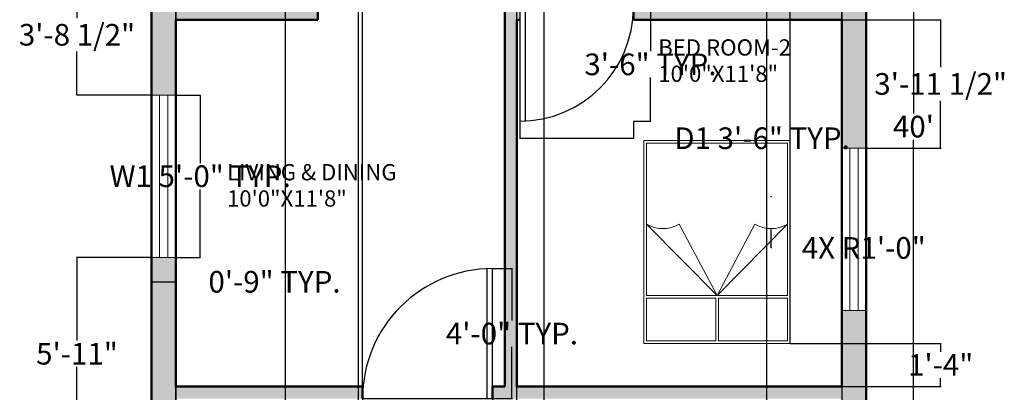
# Model space of a CAD drawing. Units: inches. Extents: x 23 to 387, y 67 to 650.
# Tile 2 of 3: x 23 to 387, y 272 to 410. Entities that reach past the tile are written whole.
import ezdxf

# ---------------------------------------------------------------- set-up
doc = ezdxf.new("R2010")
doc.units = ezdxf.units.IN
doc.header["$MEASUREMENT"] = 0
for name, color, linetype, lineweight in [('A-ANNO-DIMS', 4, 'Continuous', 18), ('A-AREA-IDEN', 4, 'Continuous', 25), ('A-DOOR', 41, 'Continuous', 25), ('A-FURN', 31, 'Continuous', 18), ('A-GLAZ', 146, 'Continuous', 18), ('A-WALL', 240, 'Continuous', 50), ('A-WALL-PATT', 31, 'Continuous', 13)]:
    doc.layers.add(name, color=color, linetype=linetype, lineweight=lineweight)
doc.styles.get("Standard").update_dxf_attribs({"font": 'italic8.shx'})
doc.dimstyles.get("Standard").update_dxf_attribs({"dimtxt": 8, "dimasz": 0.18, "dimexe": 0.18, "dimexo": 0.0625, "dimgap": 0.09, "dimtad": 0, "dimtih": 1, "dimtoh": 1, "dimdec": 1, "dimzin": 0, "dimdsep": 46, "dimlunit": 3, "dimtxsty": 'Standard', "dimcen": 0.09, "dimadec": 0, "dimazin": 0, "dimtfac": 1, "dimtdec": 1, "dimtofl": 0, "dimtmove": 0, "dimatfit": 3, "dimfxl": 1, "dimtolj": 1, "dimtzin": 0, "dimarcsym": 0})

# ---------------------------------------------------------------- blocks, each defined once
blk = doc.blocks.new('*D5')
at = {"layer": 'A-ANNO-DIMS', "color": 0, "lineweight": -2, "transparency": 16777216}
for p, q in [((335.86, 610.55), (353.42, 610.55)), ((353.24, 610.37), (353.24, 375.4)), ((353.24, 130.73), (353.24, 365.7)), ((335.86, 130.55), (353.42, 130.55))]:
    blk.add_line(p, q, dxfattribs=at)
at = {"layer": 'A-ANNO-DIMS', "color": 0, "transparency": 16777216}
for points in [[(353.21, 610.37), (353.27, 610.37), (353.24, 610.55)], [(353.21, 130.73), (353.27, 130.73), (353.24, 130.55)]]:
    blk.add_solid(points, dxfattribs=at)
at = {"layer": 'Defpoints', "color": 0, "transparency": 16777216}
for p in [(335.8, 610.55), (335.8, 130.55), (353.24, 130.55)]:
    blk.add_point(p, dxfattribs=at)
at = {"layer": 'A-ANNO-DIMS', "color": 0, "transparency": 16777216, "insert": (353.24, 370.55), "char_height": 8, "attachment_point": 5}
blk.add_mtext("\\A1;40'", dxfattribs=at)
blk = doc.blocks.new('BED-DOUBLE')
for p, q in [((26.5, 58.27), (26.5, 74)), ((27.5, 58.27), (27.5, 74)), ((1, 58.27), (26.5, 58.27)), ((27.5, 58.27), (53, 58.27)), ((1, 57.27), (53, 57.27)), ((27, 57.27), (1, 30.99)), ((13, 30.99), (27, 57.27)), ((27, 57.27), (53, 30.99)), ((41, 30.99), (27, 57.27))]:
    blk.add_line(p, q)
blk.add_lwpolyline([(54, 75), (0, 75), (0, 0), (54, 0)], close=True)
for points in [[(26.5, 74), (1, 74), (1, 58.27)], [(53, 58.27), (53, 74), (27.5, 74)], [(1, 57.27), (1, 1), (53, 1), (53, 57.27)]]:
    blk.add_lwpolyline(points)
for centre in [(7, 20.75), (47, 20.75)]:
    blk.add_arc(centre, 11.86, 59.6151, 120.3849)
blk = doc.blocks.new('DOOR-SWING-42IN')
for p, q in [((42, 42), (0, 42)), ((0, 42), (0, 0)), ((2, 42), (2, 0.05))]:
    blk.add_line(p, q)
blk.add_arc((0, 42), 42, 270, 0)
blk = doc.blocks.new('DOOR-SWING-48IN')
for p, q in [((46, 0), (46, 47.96)), ((48, 0), (48, 48)), ((0, 0), (48, 0))]:
    blk.add_line(p, q)
blk.add_arc((48, 0), 48, 90, 180)
blk = doc.blocks.new('WIN-60IN')
for p, q in [((0, 0), (0, 60)), ((0, 60), (9, 60)), ((3, 0), (3, 60)), ((6, 0), (6, 60)), ((9, 60), (9, 0)), ((9, 0), (0, 0)), ((0, 0), (4.5, 0))]:
    blk.add_line(p, q)
blk = doc.blocks.new('*D12')
at = {"layer": 'A-ANNO-DIMS', "color": 0, "lineweight": -2, "transparency": 16777216}
for p, q in [((80.86, 382.2), (89.98, 382.2)), ((89.8, 382.02), (89.8, 357.05)), ((89.8, 322.38), (89.8, 347.34)), ((80.86, 322.2), (89.98, 322.2))]:
    blk.add_line(p, q, dxfattribs=at)
at = {"layer": 'A-ANNO-DIMS', "color": 0, "transparency": 16777216}
for points in [[(89.77, 382.02), (89.83, 382.02), (89.8, 382.2)], [(89.77, 322.38), (89.83, 322.38), (89.8, 322.2)]]:
    blk.add_solid(points, dxfattribs=at)
at = {"layer": 'Defpoints', "color": 0, "transparency": 16777216}
for p in [(80.8, 382.2), (89.8, 382.2), (80.8, 322.2)]:
    blk.add_point(p, dxfattribs=at)
at = {"layer": 'A-ANNO-DIMS', "color": 0, "transparency": 16777216, "insert": (89.8, 352.2), "char_height": 8, "attachment_point": 5}
blk.add_mtext('\\A1;W1 5\'-0" TYP.', dxfattribs=at)
blk = doc.blocks.new('*D13')
at = {"layer": 'A-ANNO-DIMS', "color": 0, "lineweight": -2, "transparency": 16777216}
for p, q in [((71.8, 322.13), (71.8, 313.02)), ((80.8, 322.13), (80.8, 313.02)), ((71.98, 313.2), (80.62, 313.2)), ((80.8, 313.2), (80.98, 313.2))]:
    blk.add_line(p, q, dxfattribs=at)
at = {"layer": 'A-ANNO-DIMS', "color": 0, "transparency": 16777216}
for points in [[(71.98, 313.23), (71.98, 313.17), (71.8, 313.2)], [(80.62, 313.23), (80.62, 313.17), (80.8, 313.2)]]:
    blk.add_solid(points, dxfattribs=at)
at = {"layer": 'Defpoints', "color": 0, "transparency": 16777216}
for p in [(71.8, 322.2), (80.8, 322.2), (80.8, 313.2)]:
    blk.add_point(p, dxfattribs=at)
at = {"layer": 'A-ANNO-DIMS', "color": 0, "transparency": 16777216, "insert": (117.26, 313.2), "char_height": 8, "attachment_point": 5}
blk.add_mtext('\\A1;0\'-9" TYP.', dxfattribs=at)
blk = doc.blocks.new('*D20')
at = {"layer": 'A-ANNO-DIMS', "color": 0, "lineweight": -2, "transparency": 16777216}
for p, q in [((207.82, 372.49), (207.82, 366.07)), ((249.82, 372.49), (249.82, 366.07)), ((208, 366.25), (249.64, 366.25)), ((249.82, 366.25), (250, 366.25))]:
    blk.add_line(p, q, dxfattribs=at)
at = {"layer": 'A-ANNO-DIMS', "color": 0, "transparency": 16777216}
for points in [[(208, 366.28), (208, 366.22), (207.82, 366.25)], [(249.64, 366.28), (249.64, 366.22), (249.82, 366.25)]]:
    blk.add_solid(points, dxfattribs=at)
at = {"layer": 'Defpoints', "color": 0, "transparency": 16777216}
for p in [(207.82, 372.55), (249.82, 372.55), (249.82, 366.25)]:
    blk.add_point(p, dxfattribs=at)
at = {"layer": 'A-ANNO-DIMS', "color": 0, "transparency": 16777216, "insert": (297.33, 366.25), "char_height": 8, "attachment_point": 5}
blk.add_mtext('\\A1;D1 3\'-6" TYP.', dxfattribs=at)
blk = doc.blocks.new('*D21')
at = {"layer": 'A-ANNO-DIMS', "color": 0, "lineweight": -2, "transparency": 16777216}
for p, q in [((249.89, 414.55), (256.3, 414.55)), ((256.12, 414.37), (256.12, 398.4)), ((256.12, 372.73), (256.12, 388.7)), ((249.89, 372.55), (256.3, 372.55))]:
    blk.add_line(p, q, dxfattribs=at)
at = {"layer": 'A-ANNO-DIMS', "color": 0, "transparency": 16777216}
for points in [[(256.09, 414.37), (256.15, 414.37), (256.12, 414.55)], [(256.09, 372.73), (256.15, 372.73), (256.12, 372.55)]]:
    blk.add_solid(points, dxfattribs=at)
at = {"layer": 'Defpoints', "color": 0, "transparency": 16777216}
for p in [(249.82, 414.55), (256.12, 414.55), (249.82, 372.55)]:
    blk.add_point(p, dxfattribs=at)
at = {"layer": 'A-ANNO-DIMS', "color": 0, "transparency": 16777216, "insert": (256.12, 393.55), "char_height": 8, "attachment_point": 5}
blk.add_mtext('\\A1;3\'-6" TYP.', dxfattribs=at)
blk = doc.blocks.new('*D22')
at = {"layer": 'A-ANNO-DIMS', "color": 0, "lineweight": -2, "transparency": 16777216}
for p, q in [((149.76, 269.99), (149.76, 262.67)), ((197.76, 269.99), (197.76, 262.67)), ((149.94, 262.85), (197.58, 262.85)), ((197.76, 262.85), (197.94, 262.85))]:
    blk.add_line(p, q, dxfattribs=at)
at = {"layer": 'A-ANNO-DIMS', "color": 0, "transparency": 16777216}
for points in [[(149.94, 262.88), (149.94, 262.82), (149.76, 262.85)], [(197.58, 262.88), (197.58, 262.82), (197.76, 262.85)]]:
    blk.add_solid(points, dxfattribs=at)
at = {"layer": 'Defpoints', "color": 0, "transparency": 16777216}
for p in [(149.76, 270.05), (197.76, 270.05), (197.76, 262.85)]:
    blk.add_point(p, dxfattribs=at)
at = {"layer": 'A-ANNO-DIMS', "color": 0, "transparency": 16777216, "insert": (246.6, 262.85), "char_height": 8, "attachment_point": 5}
blk.add_mtext('\\A1;D2 4\'-0" TYP.', dxfattribs=at)
blk = doc.blocks.new('*D23')
at = {"layer": 'A-ANNO-DIMS', "color": 0, "lineweight": -2, "transparency": 16777216}
for p, q in [((197.82, 318.05), (205.14, 318.05)), ((204.96, 317.87), (204.96, 298.9)), ((204.96, 270.23), (204.96, 289.2)), ((197.82, 270.05), (205.14, 270.05))]:
    blk.add_line(p, q, dxfattribs=at)
at = {"layer": 'A-ANNO-DIMS', "color": 0, "transparency": 16777216}
for points in [[(204.93, 317.87), (204.99, 317.87), (204.96, 318.05)], [(204.93, 270.23), (204.99, 270.23), (204.96, 270.05)]]:
    blk.add_solid(points, dxfattribs=at)
at = {"layer": 'Defpoints', "color": 0, "transparency": 16777216}
for p in [(197.76, 318.05), (204.96, 318.05), (197.76, 270.05)]:
    blk.add_point(p, dxfattribs=at)
at = {"layer": 'A-ANNO-DIMS', "color": 0, "transparency": 16777216, "insert": (204.96, 294.05), "char_height": 8, "attachment_point": 5}
blk.add_mtext('\\A1;4\'-0" TYP.', dxfattribs=at)
blk = doc.blocks.new('*D30')
at = {"layer": 'A-ANNO-DIMS', "color": 0, "lineweight": -2, "transparency": 16777216}
for p, q in [((71.74, 426.74), (44.12, 426.74)), ((44.3, 426.56), (44.3, 410.65)), ((44.3, 382.38), (44.3, 398.28)), ((71.74, 382.2), (44.12, 382.2))]:
    blk.add_line(p, q, dxfattribs=at)
at = {"layer": 'A-ANNO-DIMS', "color": 0, "transparency": 16777216}
for points in [[(44.27, 426.56), (44.33, 426.56), (44.3, 426.74)], [(44.27, 382.38), (44.33, 382.38), (44.3, 382.2)]]:
    blk.add_solid(points, dxfattribs=at)
at = {"layer": 'Defpoints', "color": 0, "transparency": 16777216}
for p in [(71.8, 426.74), (44.3, 382.2), (71.8, 382.2)]:
    blk.add_point(p, dxfattribs=at)
at = {"layer": 'A-ANNO-DIMS', "color": 0, "transparency": 16777216, "insert": (44.3, 404.47), "char_height": 8, "attachment_point": 5}
blk.add_mtext('\\A1;3\'-8 1/2"', dxfattribs=at)
blk = doc.blocks.new('*D31')
at = {"layer": 'A-ANNO-DIMS', "color": 0, "lineweight": -2, "transparency": 16777216}
for p, q in [((71.74, 322.2), (44.12, 322.2)), ((44.3, 322.02), (44.3, 291.47)), ((44.3, 251.22), (44.3, 281.76)), ((71.74, 251.04), (44.12, 251.04))]:
    blk.add_line(p, q, dxfattribs=at)
at = {"layer": 'A-ANNO-DIMS', "color": 0, "transparency": 16777216}
for points in [[(44.27, 322.02), (44.33, 322.02), (44.3, 322.2)], [(44.27, 251.22), (44.33, 251.22), (44.3, 251.04)]]:
    blk.add_solid(points, dxfattribs=at)
at = {"layer": 'Defpoints', "color": 0, "transparency": 16777216}
for p in [(71.8, 322.2), (44.3, 251.04), (71.8, 251.04)]:
    blk.add_point(p, dxfattribs=at)
at = {"layer": 'A-ANNO-DIMS', "color": 0, "transparency": 16777216, "insert": (44.3, 286.62), "char_height": 8, "attachment_point": 5}
blk.add_mtext('\\A1;5\'-11"', dxfattribs=at)
blk = doc.blocks.new('*D35')
at = {"layer": 'A-ANNO-DIMS', "color": 0, "lineweight": -2, "transparency": 16777216}
for p, q in [((326.86, 410.05), (363.48, 410.05)), ((363.3, 409.87), (363.3, 392.49)), ((363.3, 362.75), (363.3, 380.12)), ((335.86, 362.57), (363.48, 362.57))]:
    blk.add_line(p, q, dxfattribs=at)
at = {"layer": 'A-ANNO-DIMS', "color": 0, "transparency": 16777216}
for points in [[(363.27, 409.87), (363.33, 409.87), (363.3, 410.05)], [(363.27, 362.75), (363.33, 362.75), (363.3, 362.57)]]:
    blk.add_solid(points, dxfattribs=at)
at = {"layer": 'Defpoints', "color": 0, "transparency": 16777216}
for p in [(326.8, 410.05), (335.8, 362.57), (363.3, 362.57)]:
    blk.add_point(p, dxfattribs=at)
at = {"layer": 'A-ANNO-DIMS', "color": 0, "transparency": 16777216, "insert": (363.3, 386.31), "char_height": 8, "attachment_point": 5}
blk.add_mtext('\\A1;3\'-11 1/2"', dxfattribs=at)
blk = doc.blocks.new('*D37')
at = {"layer": 'A-ANNO-DIMS', "color": 0, "lineweight": -2, "transparency": 16777216}
for p, q in [((80.8, 139.61), (80.8, 638.23)), ((80.98, 638.05), (81.51, 638.05)), ((148.12, 638.05), (147.59, 638.05)), ((148.3, 139.61), (148.3, 638.23))]:
    blk.add_line(p, q, dxfattribs=at)
at = {"layer": 'A-ANNO-DIMS', "color": 0, "transparency": 16777216}
for points in [[(80.98, 638.08), (80.98, 638.02), (80.8, 638.05)], [(148.12, 638.08), (148.12, 638.02), (148.3, 638.05)]]:
    blk.add_solid(points, dxfattribs=at)
at = {"layer": 'Defpoints', "color": 0, "transparency": 16777216}
for p in [(148.3, 638.05), (80.8, 139.55), (148.3, 139.55)]:
    blk.add_point(p, dxfattribs=at)
at = {"layer": 'A-ANNO-DIMS', "color": 0, "transparency": 16777216, "insert": (114.55, 638.05), "char_height": 8, "attachment_point": 5}
blk.add_mtext('\\A1;5\'-7 1/2"', dxfattribs=at)
blk = doc.blocks.new('*D38')
at = {"layer": 'A-ANNO-DIMS', "color": 0, "lineweight": -2, "transparency": 16777216}
for p, q in [((80.8, 274.61), (80.8, 638.23)), ((80.98, 638.05), (97.28, 638.05)), ((149.58, 638.05), (133.27, 638.05)), ((149.76, 274.61), (149.76, 638.23))]:
    blk.add_line(p, q, dxfattribs=at)
at = {"layer": 'A-ANNO-DIMS', "color": 0, "transparency": 16777216}
for points in [[(80.98, 638.08), (80.98, 638.02), (80.8, 638.05)], [(149.58, 638.08), (149.58, 638.02), (149.76, 638.05)]]:
    blk.add_solid(points, dxfattribs=at)
at = {"layer": 'Defpoints', "color": 0, "transparency": 16777216}
for p in [(149.76, 638.05), (80.8, 274.55), (149.76, 274.55)]:
    blk.add_point(p, dxfattribs=at)
at = {"layer": 'A-ANNO-DIMS', "color": 0, "transparency": 16777216, "insert": (115.28, 638.05), "char_height": 8, "attachment_point": 5}
blk.add_mtext('\\A1;5\'-9"', dxfattribs=at)
blk = doc.blocks.new('*D39')
at = {"layer": 'A-ANNO-DIMS', "color": 0, "lineweight": -2, "transparency": 16777216}
for p, q in [((206.8, 192.11), (206.8, 638.23)), ((206.98, 638.05), (216.62, 638.05)), ((216.8, 192.11), (216.8, 638.23)), ((216.8, 638.05), (216.98, 638.05))]:
    blk.add_line(p, q, dxfattribs=at)
at = {"layer": 'A-ANNO-DIMS', "color": 0, "transparency": 16777216}
for points in [[(206.98, 638.08), (206.98, 638.02), (206.8, 638.05)], [(216.62, 638.08), (216.62, 638.02), (216.8, 638.05)]]:
    blk.add_solid(points, dxfattribs=at)
at = {"layer": 'Defpoints', "color": 0, "transparency": 16777216}
for p in [(216.8, 638.05), (206.8, 192.05), (216.8, 192.05)]:
    blk.add_point(p, dxfattribs=at)
at = {"layer": 'A-ANNO-DIMS', "color": 0, "transparency": 16777216, "insert": (237.64, 638.05), "char_height": 8, "attachment_point": 5}
blk.add_mtext('\\A1;0\'-10"', dxfattribs=at)
blk = doc.blocks.new('*D40')
at = {"layer": 'A-ANNO-DIMS', "color": 0, "lineweight": -2, "transparency": 16777216}
for p, q in [((80.8, 601.49), (80.8, 78.87)), ((121.14, 558.4), (121.14, 78.87)), ((80.8, 79.05), (80.62, 79.05)), ((120.96, 79.05), (80.98, 79.05))]:
    blk.add_line(p, q, dxfattribs=at)
at = {"layer": 'A-ANNO-DIMS', "color": 0, "transparency": 16777216}
for points in [[(80.98, 79.08), (80.98, 79.02), (80.8, 79.05)], [(120.96, 79.08), (120.96, 79.02), (121.14, 79.05)]]:
    blk.add_solid(points, dxfattribs=at)
at = {"layer": 'Defpoints', "color": 0, "transparency": 16777216}
for p in [(80.8, 601.55), (121.14, 558.46), (80.8, 79.05)]:
    blk.add_point(p, dxfattribs=at)
at = {"layer": 'A-ANNO-DIMS', "color": 0, "transparency": 16777216, "insert": (47.39, 79.05), "char_height": 8, "attachment_point": 5}
blk.add_mtext('\\A1;3\'-4 1/2"', dxfattribs=at)
blk = doc.blocks.new('*D42')
at = {"layer": 'A-ANNO-DIMS', "color": 0, "lineweight": -2, "transparency": 16777216}
for p, q in [((202.3, 274.61), (202.3, 638.23)), ((202.48, 638.05), (206.62, 638.05)), ((206.8, 274.61), (206.8, 638.23)), ((206.8, 638.05), (206.98, 638.05))]:
    blk.add_line(p, q, dxfattribs=at)
at = {"layer": 'A-ANNO-DIMS', "color": 0, "transparency": 16777216}
for points in [[(202.48, 638.08), (202.48, 638.02), (202.3, 638.05)], [(206.62, 638.08), (206.62, 638.02), (206.8, 638.05)]]:
    blk.add_solid(points, dxfattribs=at)
at = {"layer": 'Defpoints', "color": 0, "transparency": 16777216}
for p in [(206.8, 638.05), (202.3, 274.55), (206.8, 274.55)]:
    blk.add_point(p, dxfattribs=at)
at = {"layer": 'A-ANNO-DIMS', "color": 0, "transparency": 16777216, "insert": (240.21, 638.05), "char_height": 8, "attachment_point": 5}
blk.add_mtext('\\A1;0\'-4 1/2"', dxfattribs=at)
blk = doc.blocks.new('*D43')
at = {"layer": 'A-ANNO-DIMS', "color": 0, "lineweight": -2, "transparency": 16777216}
for p, q in [((326.8, 601.49), (326.8, 78.87)), ((298.95, 586.36), (298.95, 78.87)), ((298.95, 79.05), (298.77, 79.05)), ((326.62, 79.05), (299.13, 79.05))]:
    blk.add_line(p, q, dxfattribs=at)
at = {"layer": 'A-ANNO-DIMS', "color": 0, "transparency": 16777216}
for points in [[(299.13, 79.08), (299.13, 79.02), (298.95, 79.05)], [(326.62, 79.08), (326.62, 79.02), (326.8, 79.05)]]:
    blk.add_solid(points, dxfattribs=at)
at = {"layer": 'Defpoints', "color": 0, "transparency": 16777216}
for p in [(326.8, 601.55), (298.95, 586.43), (298.95, 79.05)]:
    blk.add_point(p, dxfattribs=at)
at = {"layer": 'A-ANNO-DIMS', "color": 0, "transparency": 16777216, "insert": (280.78, 79.05), "char_height": 8, "attachment_point": 5}
blk.add_mtext('\\A1;2\'-4"', dxfattribs=at)
blk = doc.blocks.new('*D45')
at = {"layer": 'A-ANNO-DIMS', "color": 0, "lineweight": -2, "transparency": 16777216}
for p, q in [((307.71, 638.05), (307.53, 638.05)), ((307.71, 290.5), (307.71, 638.23)), ((326.62, 638.05), (307.89, 638.05)), ((326.8, 274.61), (326.8, 638.23))]:
    blk.add_line(p, q, dxfattribs=at)
at = {"layer": 'A-ANNO-DIMS', "color": 0, "transparency": 16777216}
for points in [[(307.89, 638.08), (307.89, 638.02), (307.71, 638.05)], [(326.62, 638.08), (326.62, 638.02), (326.8, 638.05)]]:
    blk.add_solid(points, dxfattribs=at)
at = {"layer": 'Defpoints', "color": 0, "transparency": 16777216}
for p in [(307.71, 638.05), (307.71, 290.44), (326.8, 274.55)]:
    blk.add_point(p, dxfattribs=at)
at = {"layer": 'A-ANNO-DIMS', "color": 0, "transparency": 16777216, "insert": (291.25, 638.05), "char_height": 8, "attachment_point": 5}
blk.add_mtext('\\A1;1\'-7"', dxfattribs=at)
blk = doc.blocks.new('*D46')
at = {"layer": 'A-ANNO-DIMS', "color": 0, "lineweight": -2, "transparency": 16777216}
for p, q in [((307.77, 290.44), (363.48, 290.44)), ((363.3, 290.26), (363.3, 287.35)), ((363.3, 274.73), (363.3, 277.64)), ((326.86, 274.55), (363.48, 274.55))]:
    blk.add_line(p, q, dxfattribs=at)
at = {"layer": 'A-ANNO-DIMS', "color": 0, "transparency": 16777216}
for points in [[(363.27, 290.26), (363.33, 290.26), (363.3, 290.44)], [(363.27, 274.73), (363.33, 274.73), (363.3, 274.55)]]:
    blk.add_solid(points, dxfattribs=at)
at = {"layer": 'Defpoints', "color": 0, "transparency": 16777216}
for p in [(307.71, 290.44), (363.3, 290.44), (326.8, 274.55)]:
    blk.add_point(p, dxfattribs=at)
at = {"layer": 'A-ANNO-DIMS', "color": 0, "transparency": 16777216, "insert": (363.3, 282.49), "char_height": 8, "attachment_point": 5}
blk.add_mtext('\\A1;1\'-4"', dxfattribs=at)
blk = doc.blocks.new('*D50')
at = {"layer": 'A-ANNO-DIMS', "color": 0, "lineweight": -2, "transparency": 16777216}
for p, q in [((300.62, 344.69), (300.8, 344.69)), ((300.71, 344.6), (300.71, 344.78)), ((300.71, 325.71), (300.71, 332.65)), ((300.89, 325.71), (300.71, 325.71))]:
    blk.add_line(p, q, dxfattribs=at)
at = {"layer": 'A-ANNO-DIMS', "color": 0, "transparency": 16777216}
blk.add_solid([(300.74, 332.65), (300.68, 332.65), (300.71, 332.83)], dxfattribs=at)
at = {"layer": 'Defpoints', "color": 0, "transparency": 16777216}
for p in [(300.71, 344.69), (300.71, 332.83)]:
    blk.add_point(p, dxfattribs=at)
at = {"layer": 'A-ANNO-DIMS', "color": 0, "transparency": 16777216, "insert": (334.89, 325.71), "char_height": 8, "attachment_point": 5}
blk.add_mtext('\\A1;4X R1\'-0"', dxfattribs=at)

msp = doc.modelspace()

# ---------------------------------------------------------------- hatches: boundary and pattern name
at = {"layer": 'A-WALL-PATT'}
h = msp.add_hatch(color=256, dxfattribs=at)
h.dxf.hatch_style = 1
h.paths.add_polyline_path([(80.8, 601.55), (168.85, 601.55), (168.85, 610.55), (71.8, 610.55), (71.8, 559.71), (80.8, 559.71)])
h.paths.add_polyline_path([(335.8, 610.55), (198.85, 610.55), (198.85, 601.55), (202.3, 601.55), (202.3, 481.55), (202.3, 465.05), (207.59, 465.05), (207.59, 469.55), (206.8, 469.55), (206.8, 601.55), (326.8, 601.55), (326.8, 570), (331.3, 570), (335.8, 570)])
h.paths.add_polyline_path([(335.8, 510), (326.8, 510), (326.8, 469.55), (249.59, 469.55), (249.59, 465.05), (250.3, 465.05), (250.3, 461.06), (254.8, 461.06), (254.8, 465.05), (326.8, 465.05), (326.8, 455.49), (335.8, 455.49)])
h.paths.add_polyline_path([(335.8, 425.49), (326.8, 425.49), (326.8, 414.55), (254.8, 414.55), (254.8, 431.06), (250.3, 431.06), (250.3, 414.55), (249.82, 414.55), (249.82, 410.05), (326.8, 410.05), (326.8, 362.57), (335.8, 362.57)])
h.paths.add_polyline_path([(335.8, 302.57), (326.8, 302.57), (326.8, 274.55), (206.8, 274.55), (206.8, 410.05), (207.82, 410.05), (207.82, 414.55), (202.3, 414.55), (202.3, 274.55), (197.76, 274.55), (197.76, 270.05), (326.8, 270.05), (326.8, 253.25), (335.8, 253.25)])
h.paths.add_polyline_path([(335.8, 217.25), (326.8, 217.25), (326.8, 192.05), (202.3, 192.05), (202.3, 139.55), (196.3, 139.55), (196.3, 130.55), (206.8, 130.55), (206.8, 187.55), (335.8, 187.55)])
h.paths.add_polyline_path([(80.8, 203.04), (71.8, 203.04), (71.8, 130.55), (148.3, 130.55), (148.3, 139.55), (80.8, 139.55)])
h.paths.add_polyline_path([(80.8, 322.2), (71.8, 322.2), (71.8, 251.04), (80.8, 251.04), (80.8, 270.05), (149.76, 270.05), (149.76, 274.55), (80.8, 274.55)])
h.paths.add_polyline_path([(80.8, 410.05), (133.3, 410.05), (133.3, 433.95), (128.8, 433.95), (128.8, 414.55), (80.8, 414.55), (80.8, 426.74), (71.8, 426.74), (71.8, 382.2), (80.8, 382.2)])
h.paths.add_polyline_path([(133.3, 479.05), (80.8, 479.05), (80.8, 511.71), (71.8, 511.71), (71.8, 456.74), (80.8, 456.74), (80.8, 474.55), (128.8, 474.55), (128.8, 469.95), (133.3, 469.95)])
h.paths.add_polyline_path([(82.53, 419.2), (134.1, 419.2), (134.1, 429.92), (82.53, 429.92)], flags=9)

# ---------------------------------------------------------------- linework, layer by layer
at = {"layer": 'A-WALL'}
for p, q in [((71.8, 610.55), (71.8, 130.55)), ((335.8, 130.55), (335.8, 610.55)), ((133.3, 433.95), (133.3, 410.05)), ((202.3, 274.55), (202.3, 414.55)), ((249.82, 414.55), (249.82, 410.05)), ((80.8, 410.05), (133.3, 410.05)), ((80.8, 410.05), (80.8, 274.55)), ((206.8, 410.05), (207.82, 410.05)), ((206.8, 274.55), (206.8, 410.05)), ((249.82, 410.05), (326.8, 410.05)), ((326.8, 274.55), (326.8, 410.05)), ((80.8, 274.55), (149.76, 274.55)), ((149.76, 274.55), (149.76, 270.05)), ((197.76, 274.55), (197.76, 270.05)), ((197.76, 274.55), (202.3, 274.55)), ((206.8, 274.55), (326.8, 274.55))]:
    msp.add_line(p, q, dxfattribs=at)

# ---------------------------------------------------------------- block references
at = {"layer": 'A-DOOR'}
for name, p in [('DOOR-SWING-42IN', (207.82, 372.55)), ('DOOR-SWING-48IN', (149.76, 270.05))]:
    msp.add_blockref(name, p, dxfattribs=at)
at = {"layer": 'A-FURN', "rotation": 180}
msp.add_blockref('BED-DOUBLE', (307.71, 365.44), dxfattribs=at)
at = {"layer": 'A-GLAZ'}
for p in [(71.8, 322.2), (326.8, 302.57)]:
    msp.add_blockref('WIN-60IN', p, dxfattribs=at)

# ---------------------------------------------------------------- texts
at = {"layer": 'A-AREA-IDEN'}
for s, p in [('BED ROOM-2', (258.99, 396.79)), ('10\'0"X11\'8"', (258.99, 387.07)), ('LIVING & DINING', (99.71, 350.69)), ('10\'0"X11\'8"', (99.71, 340.98))]:
    msp.add_text(s, height=6, dxfattribs=at).set_placement(p)

# ---------------------------------------------------------------- dimensions: what is measured, and where the dimension line sits
at = {"layer": 'A-ANNO-DIMS'}
for base, p1, p2, picture, middle in [((148.3, 638.05), (80.8, 139.55), (148.3, 139.55), '*D37', (114.55, 638.05)), ((206.8, 638.05), (202.3, 274.55), (206.8, 274.55), '*D42', (240.21, 638.05)), ((149.76, 638.05), (80.8, 274.55), (149.76, 274.55), '*D38', (115.28, 638.05)), ((216.8, 638.05), (206.8, 192.05), (216.8, 192.05), '*D39', (237.64, 638.05)), ((307.71, 638.05), (326.8, 274.55), (307.71, 290.44), '*D45', (291.25, 638.05)), ((80.8, 79.05), (121.14, 558.46), (80.8, 601.55), '*D40', (47.39, 79.05)), ((298.9524, 79.049), (326.7992, 601.549), (298.9524, 586.4268), '*D43', (280.7776, 79.049))]:
    dim = msp.add_linear_dim(base=base, p1=p1, p2=p2, dimstyle='Standard', override={"dimdec": 1, "dimlfac": 1, "dimrnd": 0, "dimzin": 1, "dimdsep": 46, "dimlunit": 4, "dimfrac": 2}, dxfattribs=at)
    dim.commit()
    dim.dimension.update_dxf_attribs({"geometry": picture, "text_midpoint": middle})
for base, p1, p2, override, picture, middle in [((353.24, 130.55), (335.8, 610.55), (335.8, 130.55), {"dimclrd": 0, "dimclre": 0, "dimclrt": 0}, '*D5', (353.24, 370.55)), ((44.3, 382.2), (71.8, 426.74), (71.8, 382.2), {"dimdec": 1, "dimlfac": 1, "dimrnd": 0, "dimzin": 1, "dimdsep": 46, "dimlunit": 4, "dimfrac": 2}, '*D30', (44.3, 404.47)), ((363.3, 362.57), (326.8, 410.05), (335.8, 362.57), {"dimdec": 1, "dimlfac": 1, "dimrnd": 0, "dimzin": 1, "dimdsep": 46, "dimlunit": 4, "dimfrac": 2}, '*D35', (363.3, 386.31)), ((44.3, 251.04), (71.8, 322.2), (71.8, 251.04), {"dimdec": 1, "dimlfac": 1, "dimrnd": 0, "dimzin": 1, "dimdsep": 46, "dimlunit": 4, "dimfrac": 2}, '*D31', (44.3, 286.62)), ((363.3, 290.44), (326.8, 274.55), (307.71, 290.44), {"dimdec": 1, "dimlfac": 1, "dimrnd": 0, "dimzin": 1, "dimdsep": 46, "dimlunit": 4, "dimfrac": 2}, '*D46', (363.3, 282.49))]:
    dim = msp.add_linear_dim(base=base, p1=p1, p2=p2, angle=90, dimstyle='Standard', override=override, dxfattribs=at)
    dim.commit()
    dim.dimension.update_dxf_attribs({"geometry": picture, "text_midpoint": middle})
for base, p1, p2, text, picture, middle in [((256.12, 414.55), (249.82, 372.55), (249.82, 414.55), '<> TYP.', '*D21', (256.12, 393.55)), ((89.8, 382.2), (80.8, 322.2), (80.8, 382.2), 'W1 <> TYP.', '*D12', (89.8, 352.2)), ((204.96, 318.05), (197.76, 270.05), (197.76, 318.05), '<> TYP.', '*D23', (204.96, 294.05))]:
    dim = msp.add_linear_dim(base=base, p1=p1, p2=p2, angle=90, text=text, dimstyle='Standard', override={"dimdec": 1, "dimlfac": 1, "dimrnd": 0, "dimzin": 1, "dimdsep": 46, "dimlunit": 4, "dimfrac": 2}, dxfattribs=at)
    dim.commit()
    dim.dimension.update_dxf_attribs({"geometry": picture, "text_midpoint": middle})
for base, p1, p2, text, picture, middle in [((249.82, 366.25), (207.82, 372.55), (249.82, 372.55), 'D1 <> TYP.', '*D20', (297.33, 366.25)), ((80.8, 313.2), (71.8, 322.2), (80.8, 322.2), '<> TYP.', '*D13', (117.26, 313.2)), ((197.76, 262.85), (149.76, 270.05), (197.76, 270.05), 'D2 <> TYP.', '*D22', (246.6, 262.85))]:
    dim = msp.add_linear_dim(base=base, p1=p1, p2=p2, text=text, dimstyle='Standard', override={"dimdec": 1, "dimlfac": 1, "dimrnd": 0, "dimzin": 1, "dimdsep": 46, "dimlunit": 4, "dimfrac": 2}, dxfattribs=at)
    dim.commit()
    dim.dimension.update_dxf_attribs({"geometry": picture, "text_midpoint": middle})
dim = msp.add_radius_dim(center=(300.71, 344.69), mpoint=(300.71, 332.83), text='4X <>', dimstyle='Standard', override={"dimdec": 1, "dimlfac": 1, "dimrnd": 0, "dimzin": 1, "dimdsep": 46, "dimlunit": 4, "dimfrac": 2}, dxfattribs=at)
dim.commit()
dim.dimension.update_dxf_attribs({"geometry": '*D50', "text_midpoint": (334.89, 325.71), "dimtype": 164})

doc.saveas('drawing.dxf')
